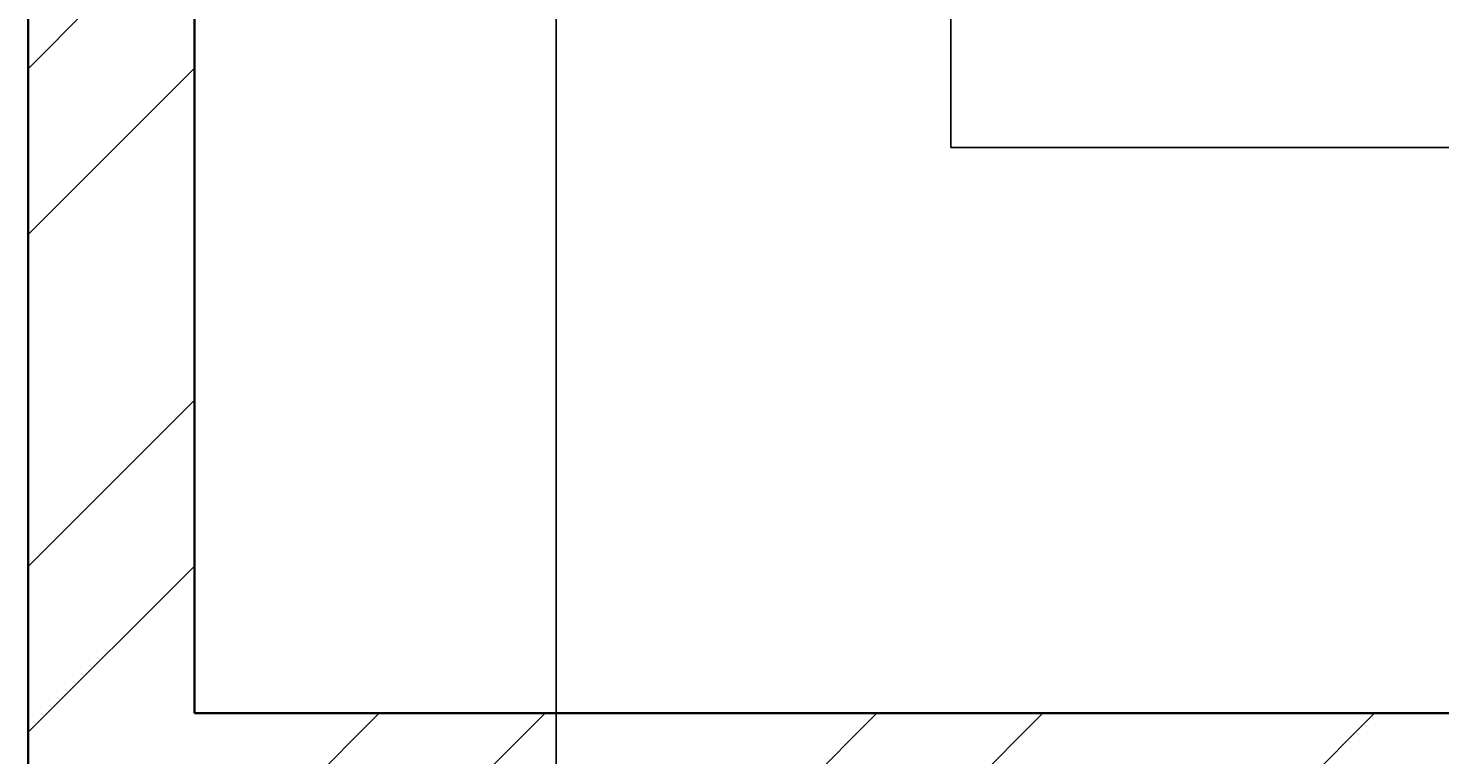
# Model space of a CAD drawing. Units: inches. Extents: x 1962 to 2771, y 1245 to 2660.
# Tile 32 of 114: x 2072 to 2110, y 1932 to 1952. Entities that reach past the tile are written whole.
import ezdxf

# ---------------------------------------------------------------- set-up
doc = ezdxf.new("R2010")
doc.units = ezdxf.units.IN
for name, color, linetype, lineweight in [('A-ANNO-DIMS', 2, 'Continuous', 18), ('A-FLOR-STRS', 7, 'Continuous', 25), ('A-WALL', 7, 'Continuous', 35), ('A-WALL-PATT', 252, 'Continuous', 13)]:
    doc.layers.add(name, color=color, linetype=linetype, lineweight=lineweight)
doc.styles.get("Standard").update_dxf_attribs({"font": 'arial.ttf'})
doc.dimstyles.get("Standard").update_dxf_attribs({"dimtxt": 0.18, "dimasz": 0.18, "dimexe": 0.18, "dimexo": 0.0625, "dimgap": 0.09, "dimtad": 0, "dimtih": 1, "dimtoh": 1, "dimdec": 4, "dimzin": 0, "dimdsep": 46, "dimtxsty": 'Standard', "dimcen": 0.09, "dimadec": 0, "dimazin": 0, "dimtfac": 1, "dimtdec": 4, "dimtofl": 0, "dimtmove": 0, "dimatfit": 3, "dimfxl": 1, "dimtolj": 1, "dimtzin": 0, "dimarcsym": 0})

# ---------------------------------------------------------------- blocks, each defined once
blk = doc.blocks.new('*D41')
at = {"layer": 'A-ANNO-DIMS', "color": 0, "lineweight": -2, "transparency": 16777216}
for p, q in [((2072.02, 1928.906), (2072.02, 1987.974)), ((2086.307, 1928.906), (2086.307, 1987.974)), ((2072.2, 1987.794), (2078.709, 1987.794)), ((2086.127, 1987.794), (2079.619, 1987.794))]:
    blk.add_line(p, q, dxfattribs=at)
at = {"layer": 'A-ANNO-DIMS', "color": 0, "transparency": 16777216}
for points in [[(2072.2, 1987.824), (2072.2, 1987.764), (2072.02, 1987.794)], [(2086.127, 1987.824), (2086.127, 1987.764), (2086.307, 1987.794)]]:
    blk.add_solid(points, dxfattribs=at)
at = {"layer": 'Defpoints', "color": 0, "transparency": 16777216}
for p in [(2086.307, 1987.794), (2072.02, 1928.844), (2086.307, 1928.844)]:
    blk.add_point(p, dxfattribs=at)
at = {"layer": 'A-ANNO-DIMS', "color": 0, "transparency": 16777216, "insert": (2079.164, 1987.794), "char_height": 0.18, "attachment_point": 5}
blk.add_mtext('\\A1;14.287', dxfattribs=at)

msp = doc.modelspace()

# ---------------------------------------------------------------- hatches: boundary and pattern name
at = {"layer": 'A-WALL-PATT'}
h = msp.add_hatch(dxfattribs=at)
h.set_pattern_fill('ANSI32', color=256)
h.paths.add_polyline_path([(2090.8074, 2467.3437), (2141.6481, 2467.3437), (2141.6481, 2469.5937), (2141.6481, 2471.8437), (2086.3074, 2471.8437), (2086.3074, 2422.5333), (2090.8074, 2422.5333)])
h.paths.add_polyline_path([(2282.7664, 2471.8437), (2204.8982, 2471.8437), (2204.8982, 2467.3437), (2234.8074, 2467.3437), (2234.8074, 2311.3437), (2228.7492, 2311.3437), (2228.7492, 2306.8437), (2234.8074, 2306.8437), (2331.9227, 2306.8437), (2331.9227, 2309.0937), (2331.9227, 2311.3437), (2239.3074, 2311.3437), (2239.3074, 2467.3437), (2282.7664, 2467.3437), (2282.7664, 2469.5937)])
h.paths.add_polyline_path([(2471.4531, 2519.8437), (2552.011, 2519.8437), (2564.3996, 2519.8437), (2564.3996, 2511.1389), (2568.8996, 2511.1389), (2568.8996, 2524.3437), (2466.9531, 2524.3437), (2466.9531, 2471.8437), (2450.0749, 2471.8437), (2446.4672, 2471.8437), (2446.4672, 2467.3437), (2450.0749, 2467.3437), (2475.9988, 2467.3437), (2475.9988, 2469.5937), (2475.9988, 2471.8437), (2471.4531, 2471.8437)])
h.paths.add_polyline_path([(2575.2231, 2469.5937), (2575.2231, 2471.8437), (2568.8996, 2471.8437), (2568.8996, 2487.1389), (2564.3996, 2487.1389), (2564.3996, 2471.8437), (2556.511, 2471.8437), (2499.2904, 2471.8437), (2499.2904, 2467.3437), (2507.8074, 2467.3437), (2507.8074, 2311.3437), (2414.863, 2311.3437), (2414.863, 2306.8437), (2512.3074, 2306.8437), (2517.0114, 2306.8437), (2517.0114, 2309.0937), (2517.0114, 2311.3437), (2512.3074, 2311.3437), (2512.3074, 2467.3437), (2575.2231, 2467.3437)])
h.paths.add_polyline_path([(2660.8074, 2471.8437), (2600.9602, 2471.8437), (2600.9602, 2467.3437), (2656.3074, 2467.3437), (2656.3074, 2432.5704), (2660.8074, 2432.5704)])
h.paths.add_polyline_path([(2660.8074, 2372.5704), (2656.3074, 2372.5704), (2656.3074, 2311.3437), (2600.276, 2311.3437), (2600.276, 2309.0937), (2600.276, 2306.8437), (2656.3074, 2306.8437), (2656.3074, 2296.2593), (2660.8074, 2296.2593)])
h.paths.add_polyline_path([(2572.3074, 2306.8437), (2577.1385, 2306.8437), (2577.1385, 2311.3437), (2551.082, 2311.3437), (2551.082, 2306.8437), (2567.8074, 2306.8437), (2567.8074, 2258.8437), (2540.0574, 2258.8437), (2540.0574, 2256.5937), (2540.0574, 2254.3437), (2567.8074, 2254.3437), (2656.3074, 2254.3437), (2656.3074, 2236.9085), (2660.8074, 2236.9085), (2660.8074, 2272.2593), (2656.3074, 2272.2593), (2656.3074, 2258.8437), (2572.3074, 2258.8437)])
h.paths.add_polyline_path([(2512.3074, 2254.3437), (2518.8716, 2254.3437), (2518.8716, 2256.5937), (2518.8716, 2258.8437), (2507.8074, 2258.8437), (2507.8074, 2177.8437), (2567.8074, 2177.8437), (2567.8074, 2172.9628), (2572.3074, 2172.9628), (2572.3074, 2177.8437), (2656.3074, 2177.8437), (2656.3074, 2166.4846), (2660.8074, 2166.4846), (2660.8074, 2200.9085), (2656.3074, 2200.9085), (2656.3074, 2182.3437), (2512.3074, 2182.3437)])
h.paths.add_polyline_path([(2656.3074, 2129.8437), (2572.3074, 2129.8437), (2572.3074, 2150.3044), (2570.0574, 2150.3044), (2567.8074, 2150.3044), (2567.8074, 2129.8437), (2507.8074, 2129.8437), (2507.8074, 2116.3027), (2510.0574, 2116.3027), (2512.3074, 2116.3027), (2512.3074, 2125.3437), (2567.8074, 2125.3437), (2572.3074, 2125.3437), (2656.3074, 2125.3437)])
h.paths.add_polyline_path([(2090.8074, 2362.5333), (2086.3074, 2362.5333), (2086.3074, 2298.6242), (2090.8074, 2298.6242), (2090.8074, 2306.8437), (2174.8074, 2306.8437), (2174.8074, 2286.4178), (2179.3074, 2286.4178), (2179.3074, 2306.8437), (2192.8641, 2306.8437), (2192.8641, 2309.0937), (2192.8641, 2311.3437), (2090.8074, 2311.3437)])
h.paths.add_polyline_path([(2209.156, 2258.8437), (2179.3074, 2258.8437), (2179.3074, 2263.2236), (2177.0574, 2263.2236), (2174.8074, 2263.2236), (2174.8074, 2258.8437), (2090.8074, 2258.8437), (2090.8074, 2274.6242), (2086.3074, 2274.6242), (2086.3074, 2238.2967), (2088.5574, 2238.2967), (2090.8074, 2238.2967), (2090.8074, 2254.3437), (2209.156, 2254.3437)])
h.paths.add_polyline_path([(2090.8074, 2177.8437), (2234.8074, 2177.8437), (2234.8074, 2173.1428), (2239.3074, 2173.1428), (2239.3074, 2258.8437), (2230.8442, 2258.8437), (2230.8442, 2256.5937), (2230.8442, 2254.3437), (2234.8074, 2254.3437), (2234.8074, 2182.3437), (2090.8074, 2182.3437), (2090.8074, 2202.2967), (2086.3074, 2202.2967), (2086.3074, 2140.0389), (2090.8074, 2140.0389)])
h.paths.add_polyline_path([(2090.8074, 2080.0389), (2086.3074, 2080.0389), (2086.3074, 2033.8437), (2090.8074, 2033.8437)], flags=17)
h.paths.add_polyline_path([(2244.9405, 2033.8437), (2239.3074, 2033.8437), (2239.3074, 2142.0665), (2237.2592, 2142.0665), (2234.8074, 2142.0665), (2234.8074, 2033.8437), (2090.8074, 2033.8437), (2076.5204, 2033.8437), (2072.0204, 2033.8437), (2072.0204, 2000.4493), (2076.5204, 2000.4493), (2076.5204, 2029.3437), (2090.8074, 2029.3437), (2244.9405, 2029.3437), (2244.9405, 2031.5937)])
h.paths.add_polyline_path([(2234.8074, 1933.3437), (2076.5204, 1933.3437), (2076.5204, 1952.4493), (2074.2704, 1952.4493), (2072.0204, 1952.4493), (2072.0204, 1933.3437), (2072.0204, 1928.8437), (2234.8074, 1928.8437)])
h.paths.add_polyline_path([(2090.8074, 1928.8437), (2086.3074, 1928.8437), (2086.3074, 1906.5013), (2090.8074, 1906.5013)])
h.paths.add_polyline_path([(2090.8074, 1846.5013), (2086.3074, 1846.5013), (2086.3074, 1769.9917), (2088.5574, 1769.9917), (2090.8074, 1769.9917), (2090.8074, 1780.3437), (2234.8074, 1780.3437), (2234.8074, 1708.3437), (2230.3764, 1708.3437), (2230.3764, 1703.8437), (2239.3074, 1703.8437), (2239.3074, 1792.6669), (2237.0574, 1792.6669), (2234.8074, 1792.6669), (2234.8074, 1784.8437), (2090.8074, 1784.8437)])
h.paths.add_polyline_path([(2239.3074, 1928.8437), (2244.9405, 1928.8437), (2244.9405, 1931.0937), (2244.9405, 1933.3437), (2234.8074, 1933.3437), (2234.8074, 1928.8437), (2234.8074, 1825.5949), (2239.3074, 1825.5949)])
h.paths.add_polyline_path([(2148.0425, 1649.0937), (2148.0425, 1651.3437), (2090.8074, 1651.3437), (2090.8074, 1646.8437), (2148.0425, 1646.8437)], flags=0)
h.paths.add_polyline_path([(2207.5601, 1708.3437), (2090.8074, 1708.3437), (2090.8074, 1703.8437), (2174.8074, 1703.8437), (2174.8074, 1651.3437), (2170.4457, 1651.3437), (2170.4457, 1646.8437), (2195.9924, 1646.8437), (2195.9924, 1649.0937), (2195.9924, 1651.3437), (2179.3074, 1651.3437), (2179.3074, 1703.8437), (2207.5601, 1703.8437), (2207.5601, 1706.0937)])
h.paths.add_polyline_path([(2090.8074, 1733.9917), (2086.3074, 1733.9917), (2086.3074, 1696.1032), (2088.5574, 1696.1032), (2090.8074, 1696.1032)])
h.paths.add_polyline_path([(2090.8074, 1672.1032), (2086.3074, 1672.1032), (2086.3074, 1600.3335), (2090.8074, 1600.3335)])
h.paths.add_polyline_path([(2090.8074, 1540.3335), (2086.3074, 1540.3335), (2086.3074, 1486.3437), (2139.6766, 1486.3437), (2139.6766, 1490.8437), (2090.8074, 1490.8437)])
h.paths.add_polyline_path([(2302.3876, 1490.8437), (2239.3074, 1490.8437), (2239.3074, 1646.8437), (2335.9994, 1646.8437), (2335.9994, 1651.3437), (2229.884, 1651.3437), (2229.884, 1646.8437), (2234.8074, 1646.8437), (2234.8074, 1490.8437), (2202.7103, 1490.8437), (2202.7103, 1488.5937), (2202.7103, 1486.3437), (2275.0699, 1486.3437), (2275.0699, 1475.772), (2279.5699, 1475.772), (2279.5699, 1486.3437), (2302.3876, 1486.3437)])
h.paths.add_polyline_path([(2279.5699, 1451.772), (2275.0699, 1451.772), (2275.0699, 1438.3437), (2174.8074, 1438.3437), (2174.8074, 1486.3437), (2179.7922, 1486.3437), (2179.7922, 1490.8437), (2163.3585, 1490.8437), (2163.3585, 1488.5937), (2163.3585, 1486.3437), (2170.3074, 1486.3437), (2170.3074, 1433.8437), (2279.5699, 1433.8437)])
h.paths.add_polyline_path([(2427.2363, 1490.8437), (2375.8074, 1490.8437), (2375.8074, 1646.8437), (2381.6401, 1646.8437), (2381.6401, 1651.3437), (2365.887, 1651.3437), (2365.887, 1649.0937), (2365.887, 1646.8437), (2371.3074, 1646.8437), (2371.3074, 1490.8437), (2327.5627, 1490.8437), (2327.5627, 1488.5937), (2327.5627, 1486.3437), (2371.3074, 1486.3437), (2371.3074, 1433.8437), (2375.8074, 1433.8437), (2375.8074, 1486.3437), (2427.2363, 1486.3437)])
h.paths.add_polyline_path([(2512.3074, 1646.8437), (2519.4351, 1646.8437), (2519.4351, 1649.0937), (2519.4351, 1651.3437), (2507.8074, 1651.3437), (2416.0063, 1651.3437), (2416.0063, 1649.0937), (2416.0063, 1646.8437), (2507.8074, 1646.8437), (2507.8074, 1490.8437), (2497.0532, 1490.8437), (2497.0532, 1488.5937), (2497.0532, 1486.3437), (2574.9344, 1486.3437), (2574.9344, 1476.0181), (2579.4344, 1476.0181), (2579.4344, 1486.3437), (2584.4872, 1486.3437), (2584.3074, 1490.8437), (2512.3074, 1490.8437)])
h.paths.add_polyline_path([(2470.5091, 1486.3437), (2473.9767, 1486.3437), (2473.9767, 1490.8437), (2449.6605, 1490.8437), (2449.6605, 1488.5937), (2449.6605, 1486.3437), (2466.0091, 1486.3437), (2466.0091, 1433.8437), (2470.5091, 1433.8437), (2579.4344, 1433.8437), (2579.4344, 1452.0181), (2574.9344, 1452.0181), (2574.9344, 1438.3437), (2554.5091, 1438.3437), (2470.5091, 1438.3437)])
h.paths.add_polyline_path([(2656.3074, 1490.8437), (2611.86, 1490.8437), (2611.86, 1486.3437), (2656.3074, 1486.3437)])
h.paths.add_polyline_path([(2660.8074, 1532.7007), (2658.5574, 1532.7007), (2656.3074, 1532.7007), (2656.3074, 1486.3437), (2660.8074, 1486.3437)])
h.paths.add_polyline_path([(2660.8074, 1664.9663), (2656.3074, 1664.9663), (2656.3074, 1651.3437), (2602.2313, 1651.3437), (2602.2313, 1646.8437), (2656.3074, 1646.8437), (2656.3074, 1592.7007), (2660.8074, 1592.7007)])
h.paths.add_polyline_path([(2660.8074, 1724.5221), (2656.3074, 1724.5221), (2656.3074, 1703.8437), (2542.4725, 1703.8437), (2542.4725, 1699.3437), (2567.8074, 1699.3437), (2567.8074, 1651.3437), (2552.7766, 1651.3437), (2552.7766, 1649.0937), (2552.7766, 1646.8437), (2577.2878, 1646.8437), (2577.2878, 1649.0937), (2577.2878, 1651.3437), (2572.3074, 1651.3437), (2572.3074, 1699.3437), (2656.3074, 1699.3437), (2656.3074, 1688.9663), (2660.8074, 1688.9663)])
h.paths.add_polyline_path([(2660.8074, 1880.6524), (2656.3074, 1880.6524), (2656.3074, 1832.8437), (2512.3074, 1832.8437), (2512.3074, 1837.8959), (2507.8074, 1837.8959), (2507.8074, 1828.3437), (2567.8074, 1828.3437), (2567.8074, 1804.3437), (2572.3074, 1804.3437), (2572.3074, 1828.3437), (2656.3074, 1828.3437), (2656.3074, 1818.6778), (2660.8074, 1818.6778)])
h.paths.add_polyline_path([(2660.8074, 1794.6778), (2656.3074, 1794.6778), (2656.3074, 1780.3437), (2572.3074, 1780.3437), (2572.3074, 1783.0303), (2570.0574, 1783.0303), (2567.8074, 1783.0303), (2567.8074, 1780.3437), (2507.8074, 1780.3437), (2507.8074, 1699.3437), (2517.8858, 1699.3437), (2517.8858, 1701.5937), (2517.8858, 1703.8437), (2512.3074, 1703.8437), (2512.3074, 1775.8437), (2656.3074, 1775.8437), (2656.3074, 1760.5221), (2660.8074, 1760.5221)])
h.paths.add_polyline_path([(2660.8074, 1981.3437), (2660.8074, 2020.2808), (2658.5574, 2020.2808), (2656.3074, 2020.2808), (2656.3074, 1981.3437), (2512.3074, 1981.3437), (2512.3074, 2086.6996), (2507.8074, 2086.6996), (2507.8074, 1981.3437), (2375.8074, 1981.3437), (2375.8074, 1986.8505), (2373.5574, 1986.8505), (2371.3074, 1986.8505), (2371.3074, 1973.2607), (2375.8074, 1973.2607), (2375.8074, 1976.8437), (2507.8074, 1976.8437), (2507.8074, 1865.4281), (2510.0574, 1865.4281), (2512.3074, 1865.4281), (2512.3074, 1976.8437), (2660.8074, 1976.8437)])
h.paths.add_polyline_path([(2375.8074, 1940.297), (2373.5574, 1940.297), (2371.3074, 1940.297), (2371.3074, 1933.3437), (2278.4434, 1933.3437), (2278.4434, 1928.8437), (2371.3074, 1928.8437), (2371.3074, 1651.3437), (2375.8074, 1651.3437)])
h.paths.add_polyline_path([(2660.8074, 1976.8437), (2656.3074, 1976.8437), (2656.3074, 1940.6524), (2660.8074, 1940.6524)], flags=17)
h.paths.add_polyline_path([(2660.8074, 2142.4846), (2656.3074, 2142.4846), (2656.3074, 2080.2808), (2660.8074, 2080.2808)])
h.paths.add_polyline_path([(2381.4189, 2311.3437), (2375.8074, 2311.3437), (2375.8074, 2467.3437), (2424.7242, 2467.3437), (2424.7242, 2469.5937), (2424.7242, 2471.8437), (2375.8074, 2471.8437), (2375.8074, 2524.3437), (2371.3074, 2524.3437), (2371.3074, 2471.8437), (2307.2097, 2471.8437), (2307.2097, 2467.3437), (2371.3074, 2467.3437), (2371.3074, 2311.3437), (2366.8901, 2311.3437), (2366.8901, 2306.8437), (2371.3074, 2306.8437), (2371.3074, 2033.8437), (2279.6589, 2033.8437), (2279.6589, 2029.3437), (2371.3074, 2029.3437), (2371.3074, 2014.2598), (2375.8074, 2014.2598), (2375.8074, 2306.8437), (2381.4189, 2306.8437)])
h.paths.add_polyline_path([(2263.3074, 2524.3437), (2170.3074, 2524.3437), (2170.3074, 2519.8437), (2170.3074, 2471.8437), (2165.0312, 2471.8437), (2165.0312, 2467.3437), (2179.6721, 2467.3437), (2179.6721, 2469.5161), (2179.6721, 2471.8437), (2174.8074, 2471.8437), (2174.8074, 2519.8437), (2258.8074, 2519.8437), (2258.8074, 2511.6436), (2263.3074, 2511.6436)])
h.paths.add_polyline_path([(2245.0232, 1361.4123), (2492.9468, 1361.4123), (2492.9468, 1398.505), (2245.0232, 1398.505)], flags=9)
h.paths.add_polyline_path([(2388.1434, 2086.6936), (2425.0704, 2086.6936), (2425.0704, 2105.3509), (2388.1434, 2105.3509)], flags=9)
h.paths.add_polyline_path([(2404.922, 2242.6744), (2445.7337, 2242.6744), (2445.7337, 2261.3318), (2404.922, 2261.3318)], flags=9)
h.paths.add_polyline_path([(2269.4107, 2156.7935), (2306.3378, 2156.7935), (2306.3378, 2175.4508), (2269.4107, 2175.4508)], flags=9)
h.paths.add_polyline_path([(2269.3277, 2233.4343), (2306.2547, 2233.4343), (2306.2547, 2252.0917), (2269.3277, 2252.0917)], flags=9)
h.paths.add_polyline_path([(2431.6052, 2320.6922), (2470.4456, 2320.6922), (2470.4456, 2339.3495), (2431.6052, 2339.3495)], flags=25)
h.paths.add_polyline_path([(2249.6902, 2315.7608), (2288.5306, 2315.7608), (2288.5306, 2334.4182), (2249.6902, 2334.4182)], flags=25)
h.paths.add_polyline_path([(2096.9301, 2314.3181), (2135.7704, 2314.3181), (2135.7704, 2332.9755), (2096.9301, 2332.9755)], flags=25)
h.paths.add_polyline_path([(2134.3475, 2285.7089), (2161.4655, 2285.7089), (2161.4655, 2304.3662), (2134.3475, 2304.3662)], flags=9)
h.paths.add_polyline_path([(2126.5155, 2209.4076), (2159.9227, 2209.4076), (2159.9227, 2228.065), (2126.5155, 2228.065)], flags=25)
h.paths.add_polyline_path([(2110.5753, 2141.5299), (2149.4157, 2141.5299), (2149.4157, 2160.1872), (2110.5753, 2160.1872)], flags=25)
h.paths.add_polyline_path([(2249.8618, 1968.3317), (2286.3966, 1968.3317), (2286.3966, 1986.989), (2249.8618, 1986.989)], flags=9)
h.paths.add_polyline_path([(2395.9507, 1777.0051), (2436.7624, 1777.0051), (2436.7624, 1795.6625), (2395.9507, 1795.6625)], flags=9)
h.paths.add_polyline_path([(2398.5259, 1888.5651), (2435.0062, 1888.5651), (2435.0062, 1907.2224), (2398.5259, 1907.2224)], flags=25)
h.paths.add_polyline_path([(2259.3506, 1728.3559), (2296.2776, 1728.3559), (2296.2776, 1747.0132), (2259.3506, 1747.0132)], flags=9)
h.paths.add_polyline_path([(2271.3698, 1845.268), (2308.2968, 1845.268), (2308.2968, 1863.9253), (2271.3698, 1863.9253)], flags=9)
h.paths.add_polyline_path([(2120.9355, 1786.3027), (2159.7759, 1786.3027), (2159.7759, 1804.9601), (2120.9355, 1804.9601)], flags=25)
h.paths.add_polyline_path([(2121.3164, 1732.1043), (2154.7236, 1732.1043), (2154.7236, 1750.7616), (2121.3164, 1750.7616)], flags=25)
h.paths.add_polyline_path([(2118.3706, 1678.8997), (2147.5282, 1678.8997), (2147.5282, 1697.557), (2118.3706, 1697.557)], flags=25)
h.paths.add_polyline_path([(2385.9227, 1493.557), (2424.763, 1493.557), (2424.763, 1512.2143), (2385.9227, 1512.2143)], flags=25)
h.paths.add_polyline_path([(2248.7058, 1500.0256), (2287.5462, 1500.0256), (2287.5462, 1518.6829), (2248.7058, 1518.6829)], flags=25)
h.paths.add_polyline_path([(2104.1669, 1617.3771), (2143.0073, 1617.3771), (2143.0073, 1636.0344), (2104.1669, 1636.0344)], flags=9)
h.paths.add_polyline_path([(2096.0714, 1447.8824), (2137.3845, 1447.8824), (2137.3845, 1458.1859), (2096.0714, 1458.1859)], flags=9)
h.paths.add_polyline_path([(2180.6114, 1440.325), (2209.7689, 1440.325), (2209.7689, 1458.9823), (2180.6114, 1458.9823)], flags=25)
h.paths.add_polyline_path([(2316.1698, 1447.9637), (2357.4829, 1447.9637), (2357.4829, 1458.2673), (2316.1698, 1458.2673)], flags=9)
h.paths.add_polyline_path([(2397.6187, 1447.9637), (2438.9318, 1447.9637), (2438.9318, 1458.2673), (2397.6187, 1458.2673)], flags=9)
h.paths.add_polyline_path([(2473.0778, 1439.5953), (2502.2354, 1439.5953), (2502.2354, 1458.2527), (2473.0778, 1458.2527)], flags=25)
h.paths.add_polyline_path([(2589.7027, 1447.8819), (2631.0158, 1447.8819), (2631.0158, 1458.1855), (2589.7027, 1458.1855)], flags=9)
h.paths.add_polyline_path([(2522.4009, 1497.5285), (2561.2413, 1497.5285), (2561.2413, 1516.1859), (2522.4009, 1516.1859)], flags=25)
h.paths.add_polyline_path([(2579.6565, 1671.3482), (2608.8141, 1671.3482), (2608.8141, 1690.0056), (2579.6565, 1690.0056)], flags=25)
h.paths.add_polyline_path([(2544.7038, 1725.5064), (2578.1111, 1725.5064), (2578.1111, 1744.1637), (2544.7038, 1744.1637)], flags=25)
h.paths.add_polyline_path([(2578.1191, 1807.472), (2607.2766, 1807.472), (2607.2766, 1826.1293), (2578.1191, 1826.1293)], flags=25)
h.paths.add_polyline_path([(2595.0614, 1835.1839), (2633.9018, 1835.1839), (2633.9018, 1853.8413), (2595.0614, 1853.8413)], flags=25)
h.paths.add_polyline_path([(2567.0097, 2097.7035), (2605.8501, 2097.7035), (2605.8501, 2116.3609), (2567.0097, 2116.3609)], flags=9)
h.paths.add_polyline_path([(2586.644, 2134.6454), (2615.8015, 2134.6454), (2615.8015, 2153.3027), (2586.644, 2153.3027)], flags=9)
h.paths.add_polyline_path([(2544.6185, 2212.6783), (2578.0258, 2212.6783), (2578.0258, 2231.3356), (2544.6185, 2231.3356)], flags=25)
h.paths.add_polyline_path([(2577.0273, 2256.9023), (2606.1849, 2256.9023), (2606.1849, 2275.5597), (2577.0273, 2275.5597)], flags=24)
h.paths.add_polyline_path([(2605.2683, 2315.2821), (2644.1087, 2315.2821), (2644.1087, 2333.9395), (2605.2683, 2333.9395)], flags=25)
h.paths.add_polyline_path([(2583.1244, 2496.1815), (2624.4375, 2496.1815), (2624.4375, 2506.4851), (2583.1244, 2506.4851)], flags=9)
h.paths.add_polyline_path([(2474.761, 2497.0823), (2503.9185, 2497.0823), (2503.9185, 2515.7397), (2474.761, 2515.7397)], flags=25)
h.paths.add_polyline_path([(2387.5787, 2494.2563), (2428.902, 2494.2563), (2428.902, 2504.5598), (2387.5787, 2504.5598)], flags=9)
h.paths.add_polyline_path([(2300.1657, 2500.1564), (2341.4788, 2500.1564), (2341.4788, 2510.46), (2300.1657, 2510.46)], flags=25)
h.paths.add_polyline_path([(2176.8589, 2497.5843), (2206.0165, 2497.5843), (2206.0165, 2516.2416), (2176.8589, 2516.2416)], flags=25)
h.paths.add_polyline_path([(2097.4668, 2494.9762), (2138.7799, 2494.9762), (2138.7799, 2505.2798), (2097.4668, 2505.2798)], flags=9)

# ---------------------------------------------------------------- linework, layer by layer
at = {"layer": 'A-FLOR-STRS'}
for p, q in [((2096.9843, 2000.646), (2096.9843, 1948.6514)), ((2096.9843, 1948.6514), (2138.0955, 1948.6514))]:
    msp.add_line(p, q, dxfattribs=at)
at = {"layer": 'A-WALL'}
for p, q in [((2072.0204, 2033.8437), (2072.0204, 1933.3437)), ((2076.5204, 2029.3437), (2076.5204, 1933.3437)), ((2072.0204, 1933.3437), (2072.0204, 1928.8437)), ((2076.5204, 1933.3437), (2244.9405, 1933.3437))]:
    msp.add_line(p, q, dxfattribs=at)

# ---------------------------------------------------------------- dimensions: what is measured, and where the dimension line sits
at = {"layer": 'A-ANNO-DIMS'}
dim = msp.add_linear_dim(base=(2086.3074, 1987.7937), p1=(2072.0204, 1928.8437), p2=(2086.3074, 1928.8437), dimstyle='Standard', override={"dimdec": 3, "dimlfac": 1, "dimrnd": 0, "dimzin": 0, "dimdsep": 46, "dimlunit": 2}, dxfattribs=at)
dim.commit()
dim.dimension.update_dxf_attribs({"geometry": '*D41', "text_midpoint": (2079.1639, 1987.7937)})

doc.saveas('drawing.dxf')
